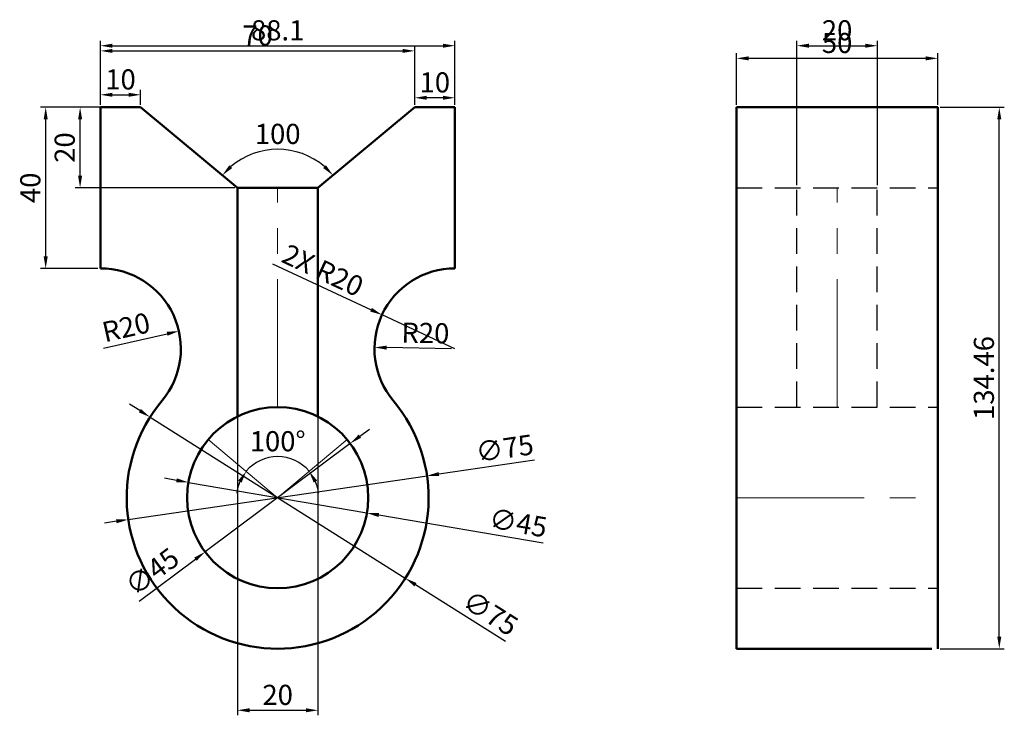
# Model space of a CAD drawing. Units: millimetres. Extents: x 24 to 269, y -6 to 167.
import ezdxf

# ---------------------------------------------------------------- set-up
doc = ezdxf.new("R2010")
doc.units = ezdxf.units.MM
doc.linetypes.add('CENTER', pattern=[50.8, 31.75, -6.35, 6.35, -6.35])
doc.linetypes.add('HIDDEN', pattern=[9.525, 6.35, -3.175])
for name, color, linetype, lineweight in [('M-CNTR', 4, 'CENTER', 18), ('M-CONS', 8, 'Continuous', 18), ('M-DIMS', 2, 'Continuous', 25), ('M-HIDN', 3, 'HIDDEN', 25), ('M-OUTL', 7, 'Continuous', 50)]:
    doc.layers.add(name, color=color, linetype=linetype, lineweight=lineweight)
doc.styles.get("Standard").update_dxf_attribs({"font": 'arial.ttf'})
doc.dimstyles.new('ISO-25', dxfattribs={"dimtxt": 5, "dimasz": 3, "dimexe": 1.25, "dimexo": 0.625, "dimtad": 1, "dimtxsty": 'Standard', "dimcen": 2.5, "dimadec": 0, "dimazin": 0, "dimtfac": 1, "dimtmove": 0, "dimatfit": 3, "dimfxl": 1, "dimarcsym": 0})

# ---------------------------------------------------------------- blocks, each defined once
blk = doc.blocks.new('*D1')
at = {"layer": 'Defpoints', "color": 0, "transparency": 16777216}
for p in [(59.38, 71.91), (116.83, 71.91), (91.03, 57.58), (88.11, 47.8), (88.11, 47.8)]:
    blk.add_point(p, dxfattribs=at)
at = {"layer": 'M-DIMS', "color": 0, "lineweight": -2, "transparency": 16777216}
for start, end in [(40, 140), (156.9086, 173.8172), (6.1828, 23.0914)]:
    blk.add_arc((88.11, 47.8), 10.2, start, end, dxfattribs=at)
at = {"layer": 'M-DIMS', "color": 0, "transparency": 16777216}
for points in [[(78.29, 52.07), (79.15, 51.54), (80.29, 54.36)], [(97.06, 51.54), (97.92, 52.07), (95.92, 54.36)]]:
    blk.add_solid(points, dxfattribs=at)
at = {"layer": 'M-DIMS', "color": 0, "transparency": 16777216, "insert": (88.11, 61.18), "char_height": 5, "attachment_point": 5}
blk.add_mtext('100°', dxfattribs=at)
blk = doc.blocks.new('*D2')
at = {"layer": 'Defpoints', "color": 0, "transparency": 16777216}
for p in [(122.15, 147.13), (122.15, 144.76), (132.15, 144.76)]:
    blk.add_point(p, dxfattribs=at)
at = {"layer": 'M-DIMS', "color": 0, "lineweight": -2, "transparency": 16777216}
for p, q in [((122.15, 145.39), (122.15, 148.38)), ((129.15, 147.13), (125.15, 147.13)), ((132.15, 145.39), (132.15, 148.38))]:
    blk.add_line(p, q, dxfattribs=at)
at = {"layer": 'M-DIMS', "color": 0, "transparency": 16777216}
for points in [[(125.15, 147.63), (125.15, 146.63), (122.15, 147.13)], [(129.15, 147.63), (129.15, 146.63), (132.15, 147.13)]]:
    blk.add_solid(points, dxfattribs=at)
at = {"layer": 'M-DIMS', "color": 0, "transparency": 16777216, "insert": (127.15, 150.3), "char_height": 5, "attachment_point": 5}
blk.add_mtext('10', dxfattribs=at)
blk = doc.blocks.new('*D3')
at = {"layer": 'Defpoints', "color": 0, "transparency": 16777216}
for p in [(54.06, 147.87), (44.06, 144.76), (54.06, 144.76)]:
    blk.add_point(p, dxfattribs=at)
at = {"layer": 'M-DIMS', "color": 0, "lineweight": -2, "transparency": 16777216}
for p, q in [((44.06, 145.39), (44.06, 149.12)), ((47.06, 147.87), (51.06, 147.87)), ((54.06, 145.39), (54.06, 149.12))]:
    blk.add_line(p, q, dxfattribs=at)
at = {"layer": 'M-DIMS', "color": 0, "transparency": 16777216}
for points in [[(47.06, 148.37), (47.06, 147.37), (44.06, 147.87)], [(51.06, 148.37), (51.06, 147.37), (54.06, 147.87)]]:
    blk.add_solid(points, dxfattribs=at)
at = {"layer": 'M-DIMS', "color": 0, "transparency": 16777216, "insert": (49.06, 151.04), "char_height": 5, "attachment_point": 5}
blk.add_mtext('10', dxfattribs=at)
blk = doc.blocks.new('*D4')
at = {"layer": 'Defpoints', "color": 0, "transparency": 16777216}
for p in [(122.15, 158.77), (44.06, 144.76), (122.15, 144.76)]:
    blk.add_point(p, dxfattribs=at)
at = {"layer": 'M-DIMS', "color": 0, "lineweight": -2, "transparency": 16777216}
for p, q in [((44.06, 145.39), (44.06, 160.02)), ((122.15, 145.39), (122.15, 160.02)), ((47.06, 158.77), (119.15, 158.77))]:
    blk.add_line(p, q, dxfattribs=at)
at = {"layer": 'M-DIMS', "color": 0, "transparency": 16777216}
for points in [[(47.06, 159.27), (47.06, 158.27), (44.06, 158.77)], [(119.15, 159.27), (119.15, 158.27), (122.15, 158.77)]]:
    blk.add_solid(points, dxfattribs=at)
at = {"layer": 'M-DIMS', "color": 0, "transparency": 16777216, "insert": (83.11, 161.95), "char_height": 5, "attachment_point": 5}
blk.add_mtext('70', dxfattribs=at)
blk = doc.blocks.new('*D5')
at = {"layer": 'Defpoints', "color": 0, "transparency": 16777216}
for p in [(54.06, 144.76), (122.15, 144.76), (93.26, 133.58), (78.11, 124.76), (98.11, 124.76)]:
    blk.add_point(p, dxfattribs=at)
at = {"layer": 'M-DIMS', "color": 0, "lineweight": -2, "transparency": 16777216}
blk.add_arc((88.11, 116.45), 17.89, 49.3699, 130.6301, dxfattribs=at)
at = {"layer": 'M-DIMS', "color": 0, "transparency": 16777216}
for points in [[(76.81, 129.67), (76.1, 130.37), (74.35, 127.88)], [(100.11, 130.37), (99.4, 129.67), (101.86, 127.88)]]:
    blk.add_solid(points, dxfattribs=at)
at = {"layer": 'M-DIMS', "color": 0, "transparency": 16777216, "insert": (88.11, 137.51), "char_height": 5, "attachment_point": 5}
blk.add_mtext('100', dxfattribs=at)
blk = doc.blocks.new('*D6')
at = {"layer": 'Defpoints', "color": 0, "transparency": 16777216}
for p in [(39.02, 144.76), (54.06, 144.76), (78.11, 124.76)]:
    blk.add_point(p, dxfattribs=at)
at = {"layer": 'M-DIMS', "color": 0, "lineweight": -2, "transparency": 16777216}
for p, q in [((53.43, 144.76), (37.77, 144.76)), ((39.02, 127.76), (39.02, 141.76)), ((77.48, 124.76), (37.77, 124.76))]:
    blk.add_line(p, q, dxfattribs=at)
at = {"layer": 'M-DIMS', "color": 0, "transparency": 16777216}
for points in [[(38.52, 141.76), (39.52, 141.76), (39.02, 144.76)], [(38.52, 127.76), (39.52, 127.76), (39.02, 124.76)]]:
    blk.add_solid(points, dxfattribs=at)
at = {"layer": 'M-DIMS', "color": 0, "transparency": 16777216, "insert": (35.84, 134.76), "char_height": 5, "attachment_point": 5, "rotation": 90}
blk.add_mtext('20', dxfattribs=at)
blk = doc.blocks.new('*D7')
at = {"layer": 'Defpoints', "color": 0, "transparency": 16777216}
for p in [(30.47, 144.76), (44.06, 144.76), (44.06, 104.76)]:
    blk.add_point(p, dxfattribs=at)
at = {"layer": 'M-DIMS', "color": 0, "lineweight": -2, "transparency": 16777216}
for p, q in [((43.43, 144.76), (29.22, 144.76)), ((30.47, 107.76), (30.47, 141.76)), ((43.43, 104.76), (29.22, 104.76))]:
    blk.add_line(p, q, dxfattribs=at)
at = {"layer": 'M-DIMS', "color": 0, "transparency": 16777216}
for points in [[(29.97, 141.76), (30.97, 141.76), (30.47, 144.76)], [(29.97, 107.76), (30.97, 107.76), (30.47, 104.76)]]:
    blk.add_solid(points, dxfattribs=at)
at = {"layer": 'M-DIMS', "color": 0, "transparency": 16777216, "insert": (27.29, 124.76), "char_height": 5, "attachment_point": 5, "rotation": 90}
blk.add_mtext('40', dxfattribs=at)
blk = doc.blocks.new('*D8')
at = {"layer": 'Defpoints', "color": 0, "transparency": 16777216}
for p in [(112.16, 85.12), (132.15, 84.76)]:
    blk.add_point(p, dxfattribs=at)
at = {"layer": 'M-DIMS', "color": 0, "lineweight": -2, "transparency": 16777216}
blk.add_line((131.33, 84.78), (115.16, 85.07), dxfattribs=at)
at = {"layer": 'M-DIMS', "color": 0, "transparency": 16777216}
blk.add_solid([(115.16, 85.57), (115.15, 84.57), (112.16, 85.12)], dxfattribs=at)
at = {"layer": 'M-DIMS', "color": 0, "transparency": 16777216, "insert": (124.8, 88.07), "char_height": 5, "attachment_point": 5, "rotation": 358.9732}
blk.add_mtext('R20', dxfattribs=at)
blk = doc.blocks.new('*D9')
at = {"layer": 'Defpoints', "color": 0, "transparency": 16777216}
for p in [(63.56, 89.18), (44.06, 84.76)]:
    blk.add_point(p, dxfattribs=at)
at = {"layer": 'M-DIMS', "color": 0, "lineweight": -2, "transparency": 16777216}
blk.add_line((44.86, 84.94), (60.64, 88.52), dxfattribs=at)
at = {"layer": 'M-DIMS', "color": 0, "transparency": 16777216}
blk.add_solid([(60.53, 89.01), (60.75, 88.03), (63.56, 89.18)], dxfattribs=at)
at = {"layer": 'M-DIMS', "color": 0, "transparency": 16777216, "insert": (50.58, 89.5), "char_height": 5, "attachment_point": 5, "rotation": 12.7741}
blk.add_mtext('R20', dxfattribs=at)
blk = doc.blocks.new('*D10')
at = {"layer": 'Defpoints', "color": 0, "transparency": 16777216}
for p in [(65.93, 51.61), (110.28, 44)]:
    blk.add_point(p, dxfattribs=at)
at = {"layer": 'M-DIMS', "color": 0, "lineweight": -2, "transparency": 16777216}
for p, q in [((62.97, 52.11), (60.02, 52.62)), ((65.93, 51.61), (110.28, 44)), ((154.06, 36.49), (113.24, 43.49))]:
    blk.add_line(p, q, dxfattribs=at)
at = {"layer": 'M-DIMS', "color": 0, "transparency": 16777216}
for points in [[(63.06, 52.61), (62.89, 51.62), (65.93, 51.61)], [(113.32, 43.98), (113.15, 43), (110.28, 44)]]:
    blk.add_solid(points, dxfattribs=at)
at = {"layer": 'M-DIMS', "color": 0, "transparency": 16777216, "insert": (147.77, 40.93), "char_height": 5, "attachment_point": 5, "rotation": 350.2676}
blk.add_mtext('∅45', dxfattribs=at)
blk = doc.blocks.new('*D11')
at = {"layer": 'Defpoints', "color": 0, "transparency": 16777216}
for p in [(125.21, 53.24), (51, 42.37)]:
    blk.add_point(p, dxfattribs=at)
at = {"layer": 'M-DIMS', "color": 0, "lineweight": -2, "transparency": 16777216}
for p, q in [((151.94, 57.15), (128.18, 53.67)), ((51, 42.37), (125.21, 53.24)), ((48.03, 41.93), (45.06, 41.5))]:
    blk.add_line(p, q, dxfattribs=at)
at = {"layer": 'M-DIMS', "color": 0, "transparency": 16777216}
for points in [[(128.11, 54.16), (128.25, 53.18), (125.21, 53.24)], [(47.96, 42.43), (48.1, 41.44), (51, 42.37)]]:
    blk.add_solid(points, dxfattribs=at)
at = {"layer": 'M-DIMS', "color": 0, "transparency": 16777216, "insert": (144.59, 59.43), "char_height": 5, "attachment_point": 5, "rotation": 8.3302}
blk.add_mtext('∅75', dxfattribs=at)
blk = doc.blocks.new('*D12')
at = {"layer": 'Defpoints', "color": 0, "transparency": 16777216}
for p in [(202.1, 156.92), (202.1, 144.76), (252.1, 144.76)]:
    blk.add_point(p, dxfattribs=at)
at = {"layer": 'M-DIMS', "color": 0, "lineweight": -2, "transparency": 16777216}
for p, q in [((202.1, 145.39), (202.1, 158.17)), ((249.1, 156.92), (205.1, 156.92)), ((252.1, 145.39), (252.1, 158.17))]:
    blk.add_line(p, q, dxfattribs=at)
at = {"layer": 'M-DIMS', "color": 0, "transparency": 16777216}
for points in [[(205.1, 157.42), (205.1, 156.42), (202.1, 156.92)], [(249.1, 157.42), (249.1, 156.42), (252.1, 156.92)]]:
    blk.add_solid(points, dxfattribs=at)
at = {"layer": 'M-DIMS', "color": 0, "transparency": 16777216, "insert": (227.1, 160.1), "char_height": 5, "attachment_point": 5}
blk.add_mtext('50', dxfattribs=at)
blk = doc.blocks.new('*D13')
at = {"layer": 'Defpoints', "color": 0, "transparency": 16777216}
for p in [(132.15, 160.06), (44.06, 144.76), (132.15, 144.76)]:
    blk.add_point(p, dxfattribs=at)
at = {"layer": 'M-DIMS', "color": 0, "lineweight": -2, "transparency": 16777216}
for p, q in [((44.06, 145.39), (44.06, 161.31)), ((47.06, 160.06), (129.15, 160.06)), ((132.15, 145.39), (132.15, 161.31))]:
    blk.add_line(p, q, dxfattribs=at)
at = {"layer": 'M-DIMS', "color": 0, "transparency": 16777216}
for points in [[(47.06, 160.56), (47.06, 159.56), (44.06, 160.06)], [(129.15, 160.56), (129.15, 159.56), (132.15, 160.06)]]:
    blk.add_solid(points, dxfattribs=at)
at = {"layer": 'M-DIMS', "color": 0, "transparency": 16777216, "insert": (88.11, 163.24), "char_height": 5, "attachment_point": 5}
blk.add_mtext('88.1', dxfattribs=at)
blk = doc.blocks.new('*D14')
at = {"layer": 'Defpoints', "color": 0, "transparency": 16777216}
for p in [(252.1, 144.76), (267.4, 144.76), (252.1, 10.3)]:
    blk.add_point(p, dxfattribs=at)
at = {"layer": 'M-DIMS', "color": 0, "lineweight": -2, "transparency": 16777216}
for p, q in [((252.72, 144.76), (268.65, 144.76)), ((267.4, 13.3), (267.4, 141.76)), ((252.72, 10.3), (268.65, 10.3))]:
    blk.add_line(p, q, dxfattribs=at)
at = {"layer": 'M-DIMS', "color": 0, "transparency": 16777216}
for points in [[(266.9, 141.76), (267.9, 141.76), (267.4, 144.76)], [(266.9, 13.3), (267.9, 13.3), (267.4, 10.3)]]:
    blk.add_solid(points, dxfattribs=at)
at = {"layer": 'M-DIMS', "color": 0, "transparency": 16777216, "insert": (264.22, 77.53), "char_height": 5, "attachment_point": 5, "rotation": 90}
blk.add_mtext('134.46', dxfattribs=at)
blk = doc.blocks.new('*D15')
at = {"layer": 'Defpoints', "color": 0, "transparency": 16777216}
for p in [(78.11, 124.76), (98.11, 124.76), (98.11, -5)]:
    blk.add_point(p, dxfattribs=at)
at = {"layer": 'M-DIMS', "color": 0, "lineweight": -2, "transparency": 16777216}
for p, q in [((78.11, 124.14), (78.11, -6.25)), ((98.11, 124.14), (98.11, -6.25)), ((81.11, -5), (95.11, -5))]:
    blk.add_line(p, q, dxfattribs=at)
at = {"layer": 'M-DIMS', "color": 0, "transparency": 16777216}
for points in [[(81.11, -4.5), (81.11, -5.5), (78.11, -5)], [(95.11, -4.5), (95.11, -5.5), (98.11, -5)]]:
    blk.add_solid(points, dxfattribs=at)
at = {"layer": 'M-DIMS', "color": 0, "transparency": 16777216, "insert": (88.11, -1.82), "char_height": 5, "attachment_point": 5}
blk.add_mtext('20', dxfattribs=at)
blk = doc.blocks.new('*D16')
at = {"layer": 'Defpoints', "color": 0, "transparency": 16777216}
for p in [(237.1, 160.06), (217.1, 124.76), (237.1, 124.76)]:
    blk.add_point(p, dxfattribs=at)
at = {"layer": 'M-DIMS', "color": 0, "lineweight": -2, "transparency": 16777216}
for p, q in [((217.1, 125.39), (217.1, 161.31)), ((220.1, 160.06), (234.1, 160.06)), ((237.1, 125.39), (237.1, 161.31))]:
    blk.add_line(p, q, dxfattribs=at)
at = {"layer": 'M-DIMS', "color": 0, "transparency": 16777216}
for points in [[(220.1, 160.56), (220.1, 159.56), (217.1, 160.06)], [(234.1, 160.56), (234.1, 159.56), (237.1, 160.06)]]:
    blk.add_solid(points, dxfattribs=at)
at = {"layer": 'M-DIMS', "color": 0, "transparency": 16777216, "insert": (227.1, 163.24), "char_height": 5, "attachment_point": 5}
blk.add_mtext('20', dxfattribs=at)
blk = doc.blocks.new('*D17')
at = {"layer": 'Defpoints', "color": 0, "transparency": 16777216}
for p in [(114.03, 93.21), (132.15, 84.76)]:
    blk.add_point(p, dxfattribs=at)
at = {"layer": 'M-DIMS', "color": 0, "lineweight": -2, "transparency": 16777216}
for p, q in [((86.83, 105.9), (111.31, 94.48)), ((132.15, 84.76), (114.03, 93.21))]:
    blk.add_line(p, q, dxfattribs=at)
at = {"layer": 'M-DIMS', "color": 0, "transparency": 16777216}
blk.add_solid([(111.52, 94.94), (111.1, 94.03), (114.03, 93.21)], dxfattribs=at)
at = {"layer": 'M-DIMS', "color": 0, "transparency": 16777216, "insert": (99.05, 103.7), "char_height": 5, "attachment_point": 5, "rotation": 335.0007}
blk.add_mtext('2X R20', dxfattribs=at)
blk = doc.blocks.new('*D18')
at = {"layer": 'Defpoints', "color": 0, "transparency": 16777216}
for p in [(56.39, 67.82), (119.82, 27.79)]:
    blk.add_point(p, dxfattribs=at)
at = {"layer": 'M-DIMS', "color": 0, "lineweight": -2, "transparency": 16777216}
for p, q in [((53.86, 69.42), (51.32, 71.02)), ((56.39, 67.82), (119.82, 27.79)), ((144.72, 12.07), (122.35, 26.19))]:
    blk.add_line(p, q, dxfattribs=at)
at = {"layer": 'M-DIMS', "color": 0, "transparency": 16777216}
for points in [[(54.12, 69.84), (53.59, 68.99), (56.39, 67.82)], [(122.62, 26.61), (122.09, 25.76), (119.82, 27.79)]]:
    blk.add_solid(points, dxfattribs=at)
at = {"layer": 'M-DIMS', "color": 0, "transparency": 16777216, "insert": (140.62, 18.59), "char_height": 5, "attachment_point": 5, "rotation": 327.7443}
blk.add_mtext('∅75', dxfattribs=at)
blk = doc.blocks.new('*D19')
at = {"layer": 'Defpoints', "color": 0, "transparency": 16777216}
for p in [(106.13, 61.27), (70.08, 34.33)]:
    blk.add_point(p, dxfattribs=at)
at = {"layer": 'M-DIMS', "color": 0, "lineweight": -2, "transparency": 16777216}
for p, q in [((108.53, 63.07), (110.93, 64.86)), ((106.13, 61.27), (70.08, 34.33)), ((53.71, 22.09), (67.68, 32.54))]:
    blk.add_line(p, q, dxfattribs=at)
at = {"layer": 'M-DIMS', "color": 0, "transparency": 16777216}
for points in [[(108.23, 63.47), (108.83, 62.67), (106.13, 61.27)], [(67.38, 32.94), (67.98, 32.14), (70.08, 34.33)]]:
    blk.add_solid(points, dxfattribs=at)
at = {"layer": 'M-DIMS', "color": 0, "transparency": 16777216, "insert": (57.28, 28.91), "char_height": 5, "attachment_point": 5, "rotation": 36.7754}
blk.add_mtext('∅45', dxfattribs=at)

msp = doc.modelspace()

# ---------------------------------------------------------------- linework, layer by layer
at = {"layer": 'M-CNTR'}
for p, q in [((88.105, 70.302), (88.105, 124.763)), ((227.096, 70.302), (227.096, 124.763)), ((202.096, 47.802), (252.096, 47.802))]:
    msp.add_line(p, q, dxfattribs=at)
at = {"layer": 'M-CONS'}
for q in [(70.869, 62.265), (105.341, 62.265)]:
    msp.add_line((88.105, 47.802), q, dxfattribs=at)
at = {"layer": 'M-HIDN'}
for p, q in [((202.096, 124.763), (252.096, 124.763)), ((217.096, 70.302), (217.096, 124.763)), ((237.096, 70.302), (237.096, 124.763)), ((202.096, 70.302), (252.096, 70.302)), ((202.096, 70.302), (227.096, 70.302)), ((202.096, 25.302), (252.096, 25.302))]:
    msp.add_line(p, q, dxfattribs=at)
at = {"layer": 'M-OUTL'}
for p, q in [((44.058, 104.763), (44.058, 144.763)), ((44.058, 144.763), (54.058, 144.763)), ((54.058, 144.763), (78.105, 124.763)), ((122.153, 144.763), (98.105, 124.763)), ((132.153, 144.763), (122.153, 144.763)), ((132.153, 104.763), (132.153, 144.763)), ((252.096, 144.763), (202.096, 144.763)), ((202.096, 144.763), (202.096, 10.302)), ((202.096, 144.763), (202.096, 124.763)), ((252.096, 144.763), (252.096, 126.789)), ((252.096, 126.789), (252.096, 10.302)), ((88.105, 124.763), (78.105, 124.763)), ((78.105, 67.958), (78.105, 124.763)), ((83.105, 124.763), (93.105, 124.763)), ((93.105, 124.763), (98.105, 124.763)), ((98.105, 67.958), (98.105, 124.763)), ((202.096, 124.763), (202.096, 84.763)), ((202.096, 124.763), (202.096, 64.763)), ((202.096, 10.302), (250.62, 10.302))]:
    msp.add_line(p, q, dxfattribs=at)
msp.add_circle((88.105, 47.802), 22.5, dxfattribs=at)
for centre, radius, start, end in [((44.058, 84.763), 20, 320, 90), ((132.153, 84.763), 20, 90, 220), ((88.105, 47.802), 37.5, 140, 40)]:
    msp.add_arc(centre, radius, start, end, dxfattribs=at)

# ---------------------------------------------------------------- dimensions: what is measured, and where the dimension line sits
at = {"layer": 'M-DIMS'}
for base, p1, p2, override, picture, middle in [((132.153, 160.063), (44.058, 144.763), (132.153, 144.763), {"dimdec": 1, "dimlfac": 1, "dimrnd": 0, "dimzin": 0, "dimdsep": 46, "dimlunit": 2}, '*D13', (88.105, 163.241)), ((237.096, 160.063), (217.096, 124.763), (237.096, 124.763), {"dimdec": 0, "dimlfac": 1, "dimrnd": 0, "dimzin": 0, "dimdsep": 46, "dimlunit": 2}, '*D16', (227.096, 163.241)), ((202.096, 156.921), (252.096, 144.763), (202.096, 144.763), {"dimclrd": 0, "dimclre": 0, "dimclrt": 0}, '*D12', (227.096, 160.099)), ((54.058, 147.865), (44.058, 144.763), (54.058, 144.763), {"dimclrd": 0, "dimclre": 0, "dimclrt": 0}, '*D3', (49.058, 151.043)), ((122.153, 147.126), (132.153, 144.763), (122.153, 144.763), {"dimclrd": 0, "dimclre": 0, "dimclrt": 0}, '*D2', (127.153, 150.304)), ((98.105, -4.998), (78.105, 124.763), (98.105, 124.763), {"dimdec": 0, "dimlfac": 1, "dimrnd": 0, "dimzin": 0, "dimdsep": 46, "dimlunit": 2}, '*D15', (88.105, -1.82))]:
    dim = msp.add_linear_dim(base=base, p1=p1, p2=p2, dimstyle='ISO-25', override=override, dxfattribs=at)
    dim.commit()
    dim.dimension.update_dxf_attribs({"geometry": picture, "text_midpoint": middle})
dim = msp.add_linear_dim(base=(122.153, 158.77), p1=(44.058, 144.763), p2=(122.153, 144.763), text='70', dimstyle='ISO-25', override={"dimclrd": 0, "dimclre": 0, "dimclrt": 0}, dxfattribs=at)
dim.commit()
dim.dimension.update_dxf_attribs({"geometry": '*D4', "text_midpoint": (83.105, 161.948)})
for base, p1, p2, override, picture, middle in [((30.468, 144.763), (44.058, 104.763), (44.058, 144.763), {"dimclrd": 0, "dimclre": 0, "dimclrt": 0}, '*D7', (27.29, 124.763)), ((39.016, 144.763), (78.105, 124.763), (54.058, 144.763), {"dimclrd": 0, "dimclre": 0, "dimclrt": 0}, '*D6', (35.838, 134.763)), ((267.396, 144.763), (252.096, 10.302), (252.096, 144.763), {"dimdec": 2, "dimlfac": 1, "dimrnd": 0, "dimzin": 0, "dimdsep": 46, "dimlunit": 2}, '*D14', (264.217, 77.533))]:
    dim = msp.add_linear_dim(base=base, p1=p1, p2=p2, angle=90, dimstyle='ISO-25', override=override, dxfattribs=at)
    dim.commit()
    dim.dimension.update_dxf_attribs({"geometry": picture, "text_midpoint": middle})
dim = msp.add_angular_dim_2l(base=(93.261, 133.575), line1=((122.153, 144.763), (98.105, 124.763)), line2=((54.058, 144.763), (78.105, 124.763)), text='100', dimstyle='ISO-25', override={"dimclrd": 0, "dimclre": 0, "dimclrt": 0}, dxfattribs=at)
dim.commit()
dim.dimension.update_dxf_attribs({"geometry": '*D5', "text_midpoint": (88.105, 137.512)})
dim = msp.add_radius_dim(center=(132.153, 84.763), mpoint=(114.026, 93.215), text='2X <>', dimstyle='ISO-25', override={"dimdec": 0, "dimlfac": 1, "dimrnd": 0, "dimzin": 0, "dimdsep": 46, "dimlunit": 2}, dxfattribs=at)
dim.commit()
dim.dimension.update_dxf_attribs({"geometry": '*D17', "text_midpoint": (99.052, 103.704)})
for center, mpoint, picture, middle in [((44.058, 84.763), (63.563, 89.185), '*D9', (51.284, 86.401)), ((132.153, 84.763), (112.156, 85.121), '*D8', (124.744, 84.895))]:
    dim = msp.add_radius_dim(center=center, mpoint=mpoint, dimstyle='ISO-25', override={"dimclrd": 0, "dimclre": 0, "dimclrt": 0}, dxfattribs=at)
    dim.commit()
    dim.dimension.update_dxf_attribs({"geometry": picture, "text_midpoint": middle, "dimtype": 164})
for p1, p2, override, picture, middle in [((56.392, 67.816), (119.818, 27.789), {"dimdec": 0, "dimlfac": 1, "dimrnd": 0, "dimzin": 0, "dimdsep": 46, "dimlunit": 2}, '*D18', (138.846, 15.781)), ((51.001, 42.369), (125.209, 53.235), {"dimclrd": 0, "dimclre": 0, "dimclrt": 0}, '*D11', (145.07, 56.143)), ((106.127, 61.273), (70.083, 34.332), {"dimdec": 0, "dimlfac": 1, "dimrnd": 0, "dimzin": 0, "dimdsep": 46, "dimlunit": 2}, '*D19', (59.269, 26.25)), ((65.929, 51.606), (110.281, 43.999), {"dimclrd": 0, "dimclre": 0, "dimclrt": 0}, '*D10', (147.211, 37.665))]:
    dim = msp.add_diameter_dim_2p(p1=p1, p2=p2, dimstyle='ISO-25', override=override, dxfattribs=at)
    dim.commit()
    dim.dimension.update_dxf_attribs({"geometry": picture, "text_midpoint": middle, "dimtype": 163})
dim = msp.add_angular_dim_2l(base=(91.031, 57.576), line1=((88.105, 47.802), (116.832, 71.907)), line2=((88.105, 47.802), (59.378, 71.907)), dimstyle='ISO-25', override={"dimclrd": 0, "dimclre": 0, "dimclrt": 0}, dxfattribs=at)
dim.commit()
dim.dimension.update_dxf_attribs({"geometry": '*D1', "text_midpoint": (88.105, 61.183)})

doc.saveas('drawing.dxf')
